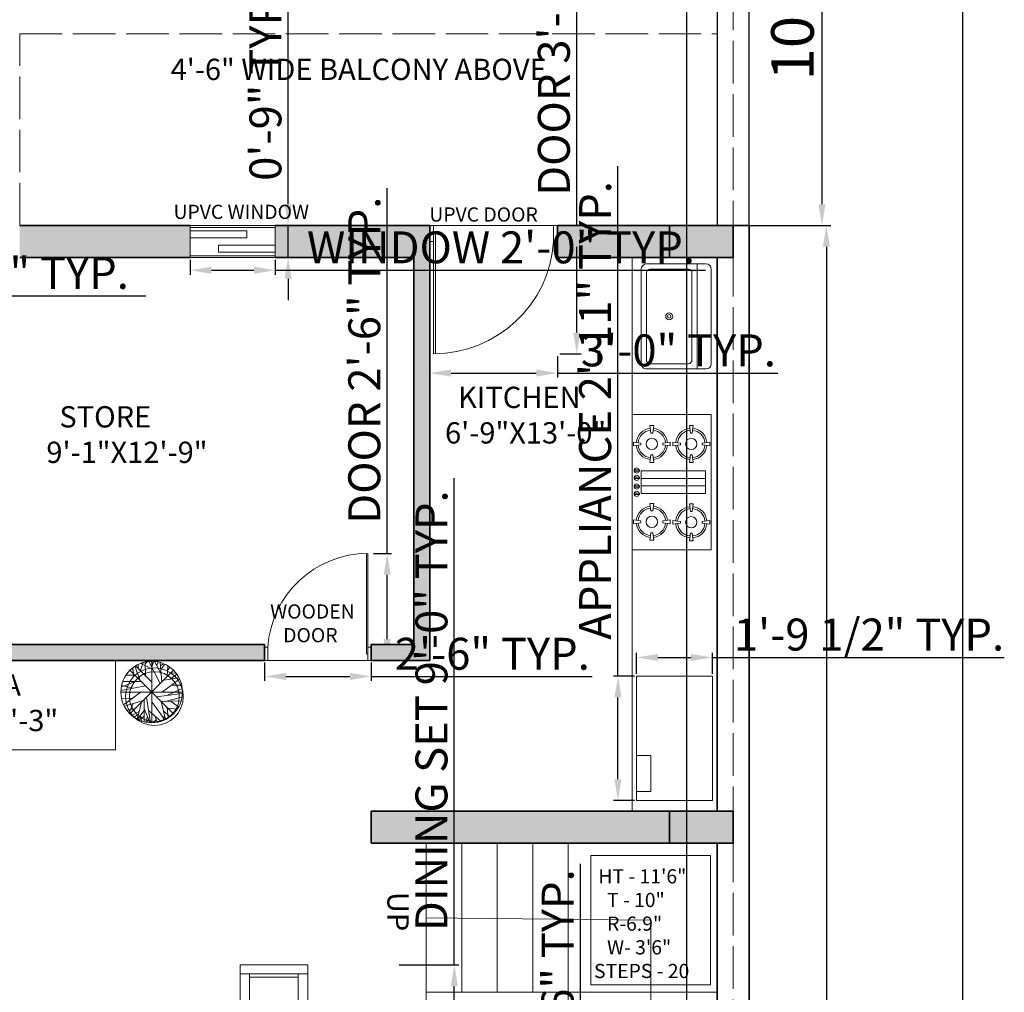
# Model space of a CAD drawing. Units: millimetres. Extents: x 595116 to 630915, y 909473 to 920225.
# Tile 125 of 134: x 629637 to 629914, y 919742 to 920016. Entities that reach past the tile are written whole.
import ezdxf

# ---------------------------------------------------------------- set-up
doc = ezdxf.new("R2010")
doc.units = ezdxf.units.MM
doc.linetypes.add('ACAD_ISO02W100', pattern=[15, 12, -3])
for name, color, linetype, lineweight in [('A-ANNO-SYMB', 7, 'Continuous', 18), ('A-AREA-IDEN', 7, 'Continuous', 20), ('A-EQPM', 8, 'Continuous', 13), ('A-FLOR-FIXT', 9, 'Continuous', 18), ('A-FLOR-OVHD', 253, 'ACAD_ISO02W100', 13), ('A-FLOR-STRS-HIDN', 142, 'ACAD_ISO02W100', 13), ('A-FURN', 32, 'Continuous', 18), ('A-WALL', 1, 'Continuous', 35), ('A-WALL-PATT', 8, 'Continuous', 13), ('C-PROP', 7, 'Continuous', 25), ('C-PROP-REF', 240, 'ACAD_ISO02W100', 13), ('Column', 6, 'Continuous', 35), ('Dimension', 3, 'Continuous', 18), ('Doors', 31, 'Continuous', 20), ('L-PLNT', 85, 'Continuous', 13), ('STAIR CASE', 142, 'Continuous', 20), ('Text', 7, 'Continuous', 18), ('Windows', 33, 'Continuous', 18)]:
    doc.layers.add(name, color=color, linetype=linetype, lineweight=lineweight)
doc.styles.get("Standard").update_dxf_attribs({"font": 'arial.ttf'})
doc.dimstyles.new('ISO-25', dxfattribs={"dimtxt": 9, "dimasz": 6, "dimexe": 1.25, "dimexo": 0.625, "dimtad": 1, "dimlunit": 4, "dimtxsty": 'Standard', "dimcen": 2.5, "dimadec": 0, "dimazin": 0, "dimtfac": 1, "dimtmove": 0, "dimatfit": 3, "dimfxl": 1, "dimarcsym": 0})

# ---------------------------------------------------------------- blocks, each defined once
blk = doc.blocks.new('KWD')
for points in [[(629753.63, 919957.93), (629752.54, 919957.93), (629752.54, 919953.43), (629753.63, 919953.43)], [(629787.45, 919957.93), (629787.45, 919953.43), (629788.54, 919953.43), (629788.54, 919957.93)]]:
    blk.add_lwpolyline(points, close=True)
blk.add_lwpolyline([(629753.63, 919921.79), (629753.63, 919955.68), (629754.13, 919955.68), (629754.13, 919921.8)])
blk.add_arc((629753.64, 919955.68), 33.88, 269.99, 356.196)
blk = doc.blocks.new('DS')
blk.add_lwpolyline([(630069.78, 919993.92), (630069.78, 919965.68), (630069.37, 919965.68), (630069.37, 919993.91)])
for points in [[(630041.6, 919963.81), (630041.6, 919967.56), (630040.69, 919967.56), (630040.69, 919963.81)], [(630069.78, 919963.81), (630070.69, 919963.81), (630070.69, 919967.56), (630069.78, 919967.56)]]:
    blk.add_lwpolyline(points, close=True)
blk.add_arc((630069.78, 919965.69), 28.24, 89.99, 176.196)
blk = doc.blocks.new('DINING')
for p, q in [((630176.61, 919568.69), (630176.61, 919601.05)), ((630176.61, 919601.05), (630208.41, 919601.05)), ((630208.41, 919601.05), (630208.41, 919568.69)), ((630176.61, 919596.78), (630208.41, 919596.78)), ((630181.05, 919571.76), (630181.05, 919596.78)), ((630181.05, 919595.21), (630203.97, 919595.21)), ((630203.97, 919571.76), (630203.97, 919596.78)), ((630176.61, 919570.82), (630180.11, 919570.82)), ((630208.41, 919570.82), (630204.91, 919570.82)), ((630163.47, 919568.69), (630222.04, 919568.69)), ((630163.47, 919453.21), (630163.47, 919568.69)), ((630164.11, 919568.05), (630221.39, 919568.05)), ((630164.11, 919453.85), (630164.11, 919568.05)), ((630221.39, 919568.05), (630221.39, 919453.85)), ((630222.04, 919568.69), (630222.04, 919453.21)), ((630163.47, 919544.57), (630135.12, 919544.57)), ((630135.12, 919544.57), (630135.12, 919519)), ((630137.93, 919544.57), (630137.93, 919519)), ((630138.72, 919544.57), (630138.72, 919519)), ((630222.04, 919544.57), (630250.39, 919544.57)), ((630246.79, 919544.57), (630246.79, 919519)), ((630247.58, 919544.57), (630247.58, 919519)), ((630250.39, 919544.57), (630250.39, 919519)), ((630135.12, 919519), (630163.47, 919519)), ((630250.39, 919519), (630222.04, 919519)), ((630163.47, 919503.52), (630135.12, 919503.52)), ((630135.12, 919503.52), (630135.12, 919477.96)), ((630137.93, 919503.52), (630137.93, 919477.96)), ((630138.72, 919503.52), (630138.72, 919477.96)), ((630222.04, 919503.52), (630250.39, 919503.52)), ((630246.79, 919503.52), (630246.79, 919477.96)), ((630247.58, 919503.52), (630247.58, 919477.96)), ((630250.39, 919503.52), (630250.39, 919477.96)), ((630135.12, 919477.96), (630163.47, 919477.96)), ((630250.39, 919477.96), (630222.04, 919477.96)), ((630222.04, 919453.21), (630163.47, 919453.21)), ((630221.39, 919453.85), (630164.11, 919453.85)), ((630176.61, 919453.21), (630176.61, 919420.86)), ((630176.61, 919451.09), (630180.11, 919451.09)), ((630208.41, 919451.09), (630204.91, 919451.09)), ((630208.41, 919420.86), (630208.41, 919453.21)), ((630181.05, 919450.14), (630181.05, 919425.13)), ((630203.97, 919450.14), (630203.97, 919425.13)), ((630176.61, 919425.13), (630208.41, 919425.13)), ((630181.05, 919426.7), (630203.97, 919426.7)), ((630176.61, 919420.86), (630208.41, 919420.86))]:
    blk.add_line(p, q)
for centre, start, end in [((630180.11, 919571.76), 270, 0), ((630204.91, 919571.76), 180, 270), ((630180.11, 919450.14), 0, 90), ((630204.91, 919450.14), 90, 180)]:
    blk.add_arc(centre, 0.945, start, end)
blk = doc.blocks.new('A$C57CF26DA')
for p, q in [((0, 0), (0, 420)), ((720, 420), (0, 420)), ((720, 0), (720, 420)), ((166.9, 413), (146.9, 413)), ((146.9, 413), (151.9, 373)), ((151.9, 373), (161.9, 373)), ((161.9, 373), (166.9, 413)), ((300, 390.9), (300, 49.1)), ((300, 390.9), (420, 390.9)), ((340, 390.9), (340, 49.1)), ((380, 390.9), (380, 49.1)), ((420, 390.9), (420, 49.1)), ((583.6, 413), (563.6, 413)), ((563.6, 413), (568.6, 373)), ((568.6, 373), (578.6, 373)), ((578.6, 373), (583.6, 413)), ((98.9, 320), (58.9, 325)), ((58.9, 325), (58.9, 305)), ((98.9, 310), (98.9, 320)), ((254.8, 325), (214.8, 320)), ((214.8, 320), (214.8, 310)), ((254.8, 305), (254.8, 325)), ((515.6, 320), (475.6, 325)), ((475.6, 325), (475.6, 305)), ((515.6, 310), (515.6, 320)), ((671.6, 325), (631.6, 320)), ((631.6, 320), (631.6, 310)), ((671.6, 305), (671.6, 325)), ((58.9, 305), (98.9, 310)), ((214.8, 310), (254.8, 305)), ((475.6, 305), (515.6, 310)), ((631.6, 310), (671.6, 305)), ((151.9, 257), (146.9, 217)), ((146.9, 217), (166.9, 217)), ((161.9, 257), (151.9, 257)), ((166.9, 217), (161.9, 257)), ((568.6, 257), (563.6, 217)), ((563.6, 217), (583.6, 217)), ((578.6, 257), (568.6, 257)), ((583.6, 217), (578.6, 257)), ((166.9, 203), (146.9, 203)), ((146.9, 203), (151.9, 163)), ((151.9, 163), (161.9, 163)), ((161.9, 163), (166.9, 203)), ((581.1, 203), (561.1, 203)), ((561.1, 203), (566.1, 163)), ((566.1, 163), (576.1, 163)), ((576.1, 163), (581.1, 203)), ((98.9, 110), (58.9, 115)), ((58.9, 115), (58.9, 95)), ((98.9, 100), (98.9, 110)), ((254.8, 115), (214.8, 110)), ((214.8, 110), (214.8, 100)), ((254.8, 95), (254.8, 115)), ((513.1, 110), (473.1, 115)), ((473.1, 115), (473.1, 95)), ((513.1, 100), (513.1, 110)), ((669, 115), (629, 110)), ((629, 110), (629, 100)), ((669, 95), (669, 115)), ((58.9, 95), (98.9, 100)), ((214.8, 100), (254.8, 95)), ((473.1, 95), (513.1, 100)), ((629, 100), (669, 95)), ((151.9, 47), (146.9, 7)), ((146.9, 7), (166.9, 7)), ((161.9, 47), (151.9, 47)), ((166.9, 7), (161.9, 47)), ((301.5, 38.7), (294.7, 38.7)), ((294.7, 38.7), (294.7, 11.3)), ((294.7, 11.3), (301.5, 11.3)), ((420, 49.1), (300, 49.1)), ((301.5, 11.3), (301.5, 38.7)), ((340.5, 38.7), (333.7, 38.7)), ((333.7, 38.7), (333.7, 11.3)), ((333.7, 11.3), (340.5, 11.3)), ((340.5, 11.3), (340.5, 38.7)), ((379.7, 11.3), (379.7, 38.7)), ((379.7, 38.7), (386.5, 38.7)), ((386.5, 11.3), (379.7, 11.3)), ((386.5, 38.7), (386.5, 11.3)), ((418.7, 11.3), (418.7, 38.7)), ((418.7, 38.7), (425.5, 38.7)), ((425.5, 11.3), (418.7, 11.3)), ((425.5, 38.7), (425.5, 11.3)), ((566.1, 47), (561.1, 7)), ((561.1, 7), (581.1, 7)), ((576.1, 47), (566.1, 47)), ((581.1, 7), (576.1, 47)), ((720, 0), (0, 0))]:
    blk.add_line(p, q)
for centre in [(156.9, 315), (573.6, 315), (156.9, 105), (571.1, 105)]:
    blk.add_circle(centre, 30)
for centre, radius, start, end in [((156.9, 315), 83, 95.5849, 174.4151), ((156.9, 315), 73, 95.3738, 174.6262), ((156.9, 315), 73, 5.3738, 84.6262), ((156.9, 315), 83, 5.5849, 84.4151), ((573.6, 315), 83, 95.5849, 174.4151), ((573.6, 315), 73, 95.3738, 174.6262), ((573.6, 315), 73, 5.3738, 84.6262), ((573.6, 315), 83, 5.5849, 84.4151), ((156.9, 315), 83, 185.5849, 264.4151), ((156.9, 315), 73, 185.3738, 264.6262), ((156.9, 315), 73, 275.3738, 354.6262), ((156.9, 315), 83, 275.5849, 354.4151), ((573.6, 315), 83, 185.5849, 264.4151), ((573.6, 315), 73, 185.3738, 264.6262), ((573.6, 315), 73, 275.3738, 354.6262), ((573.6, 315), 83, 275.5849, 354.4151), ((156.9, 105), 83, 95.5849, 174.4151), ((156.9, 105), 73, 95.3738, 174.6262), ((156.9, 105), 73, 5.3738, 84.6262), ((156.9, 105), 83, 5.5849, 84.4151), ((571.1, 105), 83, 95.5849, 174.4151), ((571.1, 105), 73, 95.3738, 174.6262), ((571.1, 105), 73, 5.3738, 84.6262), ((571.1, 105), 83, 5.5849, 84.4151), ((156.9, 105), 83, 185.5849, 264.4151), ((156.9, 105), 73, 185.3738, 264.6262), ((156.9, 105), 73, 275.3738, 354.6262), ((156.9, 105), 83, 275.5849, 354.4151), ((571.1, 105), 83, 185.5849, 264.4151), ((571.1, 105), 73, 185.3738, 264.6262), ((571.1, 105), 73, 275.3738, 354.6262), ((571.1, 105), 83, 275.5849, 354.4151), ((298.1, 25), 13.7, 104.4775, 255.5225), ((298.1, 25), 13.7, 284.4775, 75.5225), ((337.1, 25), 13.7, 104.4775, 255.5225), ((337.1, 25), 13.7, 284.4775, 75.5225), ((383.1, 25), 13.7, 104.4775, 255.5225), ((383.1, 25), 13.7, 284.4775, 75.5225), ((422.1, 25), 13.7, 104.4775, 255.5225), ((422.1, 25), 13.7, 284.4775, 75.5225)]:
    blk.add_arc(centre, radius, start, end)
blk = doc.blocks.new('Sink-single - 30 in top')
blk.add_line((-15, -3.999996), (15, -3.999996))
for points in [[(-13.5, 0), (13.5, 0)], [(-15, -18.499996), (-15, -1.5)], [(15, -1.5), (15, -18.499996)], [(-12.5, -5.499996), (12.5, -5.499996)], [(-13.5, -17.499996), (-13.5, -6.499996)], [(13.5, -6.499996), (13.5, -17.499996)], [(12.5, -18.499996), (-12.5, -18.499996)], [(13.5, -19.999996), (-13.5, -19.999996)]]:
    blk.add_lwpolyline(points)
for radius in [1, 0.5]:
    blk.add_circle((0, -11.999996), radius)
for centre, radius, start, end in [((-13.5, -1.5), 1.5, 90, 180), ((13.5, -1.5), 1.5, 0, 90), ((-12.5, -6.499996), 1, 90, 180), ((12.5, -6.499996), 1, 0, 90), ((-13.5, -18.499996), 1.5, 180, 270), ((-12.5, -17.499996), 1, 180, 270), ((12.5, -17.499996), 1, 270, 0), ((13.5, -18.499996), 1.5, 270, 0)]:
    blk.add_arc(centre, radius, start, end)
blk = doc.blocks.new('*D121')
at = {"layer": 'Defpoints', "color": 0, "transparency": 16777216}
for p in [(629838.04, 920084.93), (629838.04, 919957.93), (629863.03, 919957.93)]:
    blk.add_point(p, dxfattribs=at)
at = {"layer": 'Dimension', "color": 0, "lineweight": -2, "transparency": 16777216}
for p, q in [((629838.67, 920084.93), (629864.28, 920084.93)), ((629863.03, 920078.93), (629863.03, 919963.93)), ((629838.67, 919957.93), (629864.28, 919957.93))]:
    blk.add_line(p, q, dxfattribs=at)
at = {"layer": 'Dimension', "color": 0, "transparency": 16777216}
for points in [[(629862.03, 920078.93), (629864.03, 920078.93), (629863.03, 920084.93)], [(629862.03, 919963.93), (629864.03, 919963.93), (629863.03, 919957.93)]]:
    blk.add_solid(points, dxfattribs=at)
at = {"layer": 'Dimension', "color": 0, "transparency": 16777216, "insert": (629856.28, 920021.43), "char_height": 12, "attachment_point": 5, "rotation": 90}
blk.add_mtext('10\'-7"', dxfattribs=at)
blk = doc.blocks.new('*D122')
at = {"layer": 'Defpoints', "color": 0, "transparency": 16777216}
for p in [(629862.34, 919957.93), (629854.28, 919369.93), (629864.28, 919369.93)]:
    blk.add_point(p, dxfattribs=at)
at = {"layer": 'Dimension', "color": 0, "lineweight": -2, "transparency": 16777216}
for p, q in [((629862.97, 919957.93), (629865.53, 919957.93)), ((629864.28, 919951.93), (629864.28, 919375.93)), ((629854.9, 919369.93), (629865.53, 919369.93))]:
    blk.add_line(p, q, dxfattribs=at)
at = {"layer": 'Dimension', "color": 0, "transparency": 16777216}
for points in [[(629863.28, 919951.93), (629865.28, 919951.93), (629864.28, 919957.93)], [(629863.28, 919375.93), (629865.28, 919375.93), (629864.28, 919369.93)]]:
    blk.add_solid(points, dxfattribs=at)
at = {"layer": 'Dimension', "color": 0, "transparency": 16777216, "insert": (629857.53, 919663.93), "char_height": 12, "attachment_point": 5, "rotation": 90}
blk.add_mtext("49'", dxfattribs=at)
blk = doc.blocks.new('*D124')
at = {"layer": 'Defpoints', "color": 0, "transparency": 16777216}
for p in [(629865.75, 920084.93), (629865.75, 919141.93), (629902.57, 919141.93)]:
    blk.add_point(p, dxfattribs=at)
at = {"layer": 'Dimension', "color": 0, "lineweight": -2, "transparency": 16777216}
for p, q in [((629866.37, 920084.93), (629903.82, 920084.93)), ((629902.57, 920078.93), (629902.57, 919147.93)), ((629866.37, 919141.93), (629903.82, 919141.93))]:
    blk.add_line(p, q, dxfattribs=at)
at = {"layer": 'Dimension', "color": 0, "transparency": 16777216}
for points in [[(629901.57, 920078.93), (629903.57, 920078.93), (629902.57, 920084.93)], [(629901.57, 919147.93), (629903.57, 919147.93), (629902.57, 919141.93)]]:
    blk.add_solid(points, dxfattribs=at)
at = {"layer": 'Dimension', "color": 0, "transparency": 16777216, "insert": (629897.35, 919613.43), "char_height": 9, "attachment_point": 5, "rotation": 90}
blk.add_mtext('78\'-7"', dxfattribs=at)
blk = doc.blocks.new('POTTED-PLANT')
for p, q in [((3.96, 16.73), (5.31, 12.84)), ((4.16, 16.82), (8.64, 12.35)), ((4.85, 16.17), (4.88, 17.22)), ((5.49, 15.52), (6.28, 17.77)), ((5.61, 17.51), (8.67, 15.94)), ((6.86, 17.38), (7.52, 18.03)), ((6.89, 14.08), (6.86, 17.93)), ((7.9, 18.06), (11.06, 11.86)), ((9.02, 17.38), (8.46, 18.1)), ((8.67, 18.11), (8.67, 0.76)), ((8.74, 16.47), (9.2, 18.06)), ((11.32, 14.57), (9.46, 18.06)), ((10.09, 16.89), (10.53, 17.9)), ((11.52, 12.26), (11.04, 17.77)), ((11.14, 16.82), (12.03, 17.41)), ((11.24, 15.75), (12.36, 17.28)), ((13.25, 16.79), (13.05, 13.86)), ((1.47, 14.18), (3.93, 14.18)), ((14.75, 15.51), (2.6, 3.36)), ((14.75, 3.36), (2.6, 15.51)), ((2.87, 15.88), (3.4, 15.68)), ((3.32, 16.24), (3.58, 14.57)), ((13.17, 15.58), (13.86, 16.4)), ((13.91, 13.07), (15.74, 14.51)), ((14.04, 14.8), (15.41, 14.87)), ((0.04, 9.84), (6.94, 11.18)), ((4.01, 12.42), (0.12, 10.79)), ((0.19, 11.28), (3.48, 10.53)), ((0.57, 12.45), (5.66, 12.45)), ((16.53, 13.1), (11.7, 9.48)), ((12.05, 12.81), (16.38, 13.4)), ((14.24, 11.38), (17.09, 11.41)), ((0, 9.44), (17.35, 9.44)), ((0.78, 5.86), (5.74, 9.45)), ((10.02, 8.11), (17.3, 9.03)), ((12.92, 8.47), (17.27, 10.46)), ((0.22, 7.66), (3.4, 7.75)), ((0.98, 5.47), (6.25, 7.04)), ((3.48, 6.19), (2.31, 3.58)), ((5.79, 6.51), (4.54, 1.82)), ((6.53, 7.26), (6.56, 1.1)), ((7.22, 7.98), (8.31, 0.8)), ((8.67, 6.68), (12.41, 1.65)), ((11.37, 6.74), (12.54, 1.72)), ((11.39, 6.74), (16.97, 6.94)), ((12.49, 6.77), (17.19, 8.01)), ((14.19, 6.81), (16.25, 5.24)), ((3.99, 4.75), (1.72, 4.29)), ((5.1, 3.97), (3.07, 2.83)), ((4.88, 3.09), (3.65, 2.4)), ((6.56, 4.2), (4.67, 1.78)), ((5.56, 2.86), (5.79, 1.33)), ((6.56, 4.78), (8.11, 0.84)), ((7.78, 4.2), (11.26, 1.2)), ((11.98, 4.16), (13.78, 2.43)), ((12.26, 2.96), (12, 1.49)), ((13.07, 5.08), (13.35, 2.21)), ((13.22, 4.91), (15.85, 4.62)), ((6.56, 2.6), (5.05, 1.59)), ((7.45, 2.57), (7.01, 0.97)), ((7.75, 1.82), (7.32, 0.93)), ((9.89, 1.75), (9.23, 0.84)), ((9.53, 2.7), (10.2, 0.97))]:
    blk.add_line(p, q)
for centre, radius in [((8.67, 9.44), 8.67), ((9.43, 8.14), 8.14), ((9.43, 8.14), 7.03)]:
    blk.add_circle(centre, radius)
blk = doc.blocks.new('WIN-UPVC-2FT')
for p, q in [((0, 9), (0, 0)), ((0, 9), (24, 9)), ((24, 9), (24, 0)), ((0, 7.5), (16, 7.5)), ((0, 0), (24, 0))]:
    blk.add_line(p, q)
blk.add_lwpolyline([(0, 8.46), (24, 8.46), (24, 0.48), (0, 0.48)], close=True)
for points in [[(0, 5.5), (16, 5.5), (16, 7.5)], [(24, 1.5), (8, 1.5), (8, 3.5), (24, 3.5)]]:
    blk.add_lwpolyline(points)
blk = doc.blocks.new('KITCHEN-APPLIANCE')
for points in [[(0, 35.07), (21.33, 35.07), (21.33, 0), (0, 0)], [(0, 12.66), (4.02, 12.66), (4.02, 2.57), (0, 2.57)]]:
    blk.add_lwpolyline(points, close=True)
blk = doc.blocks.new('COLUMN-RECT-18X9')
h = blk.add_hatch(color=256)
h.dxf.hatch_style = 1
h.paths.add_polyline_path([(18, 9), (0, 9), (0, 0), (18, 0)])
blk.add_lwpolyline([(0, 9), (18, 9), (18, 0), (0, 0)], close=True)
blk = doc.blocks.new('COLUMN-RECT-18X9-B')
h = blk.add_hatch(color=256)
h.dxf.hatch_style = 1
h.paths.add_polyline_path([(18, 0), (18, 9), (0, 9), (0, 0)])
blk.add_lwpolyline([(0, 9), (18, 9), (18, 0), (0, 0)], close=True)
blk = doc.blocks.new('*D160')
at = {"layer": 'Defpoints', "color": 0, "transparency": 16777216}
for p in [(629788.54, 919957.93), (629793.96, 919957.93), (629788.54, 919921.79)]:
    blk.add_point(p, dxfattribs=at)
at = {"layer": 'Dimension', "color": 0, "lineweight": -2, "transparency": 16777216}
for p, q in [((629793.96, 919957.93), (629793.96, 920060.8)), ((629789.17, 919957.93), (629795.21, 919957.93)), ((629793.96, 919927.79), (629793.96, 919951.93)), ((629789.17, 919921.79), (629795.21, 919921.79))]:
    blk.add_line(p, q, dxfattribs=at)
at = {"layer": 'Dimension', "color": 0, "transparency": 16777216}
for points in [[(629792.96, 919951.93), (629794.96, 919951.93), (629793.96, 919957.93)], [(629792.96, 919927.79), (629794.96, 919927.79), (629793.96, 919921.79)]]:
    blk.add_solid(points, dxfattribs=at)
at = {"layer": 'Dimension', "color": 0, "transparency": 16777216, "insert": (629788.68, 920012.36), "char_height": 9, "attachment_point": 5, "rotation": 90}
blk.add_mtext('DOOR 3\'-0" TYP.', dxfattribs=at)
blk = doc.blocks.new('*D161')
at = {"layer": 'Defpoints', "color": 0, "transparency": 16777216}
for p in [(629752.54, 919921.79), (629788.54, 919921.79), (629788.54, 919916.37)]:
    blk.add_point(p, dxfattribs=at)
at = {"layer": 'Dimension', "color": 0, "lineweight": -2, "transparency": 16777216}
for p, q in [((629752.54, 919921.16), (629752.54, 919915.12)), ((629788.54, 919921.16), (629788.54, 919915.12)), ((629758.54, 919916.37), (629782.54, 919916.37)), ((629788.54, 919916.37), (629850.64, 919916.37))]:
    blk.add_line(p, q, dxfattribs=at)
at = {"layer": 'Dimension', "color": 0, "transparency": 16777216}
for points in [[(629758.54, 919917.37), (629758.54, 919915.37), (629752.54, 919916.37)], [(629782.54, 919917.37), (629782.54, 919915.37), (629788.54, 919916.37)]]:
    blk.add_solid(points, dxfattribs=at)
at = {"layer": 'Dimension', "color": 0, "transparency": 16777216, "insert": (629822.59, 919921.59), "char_height": 9, "attachment_point": 5}
blk.add_mtext('3\'-0" TYP.', dxfattribs=at)
blk = doc.blocks.new('*D164')
at = {"layer": 'Defpoints', "color": 0, "transparency": 16777216}
for p in [(629736.04, 919865.54), (629740.56, 919865.54), (629736.04, 919835.43)]:
    blk.add_point(p, dxfattribs=at)
at = {"layer": 'Dimension', "color": 0, "lineweight": -2, "transparency": 16777216}
for p, q in [((629740.56, 919865.54), (629740.56, 919968.42)), ((629736.67, 919865.54), (629741.81, 919865.54)), ((629740.56, 919841.43), (629740.56, 919859.54)), ((629736.67, 919835.43), (629741.81, 919835.43))]:
    blk.add_line(p, q, dxfattribs=at)
at = {"layer": 'Dimension', "color": 0, "transparency": 16777216}
for points in [[(629739.56, 919859.54), (629741.56, 919859.54), (629740.56, 919865.54)], [(629739.56, 919841.43), (629741.56, 919841.43), (629740.56, 919835.43)]]:
    blk.add_solid(points, dxfattribs=at)
at = {"layer": 'Dimension', "color": 0, "transparency": 16777216, "insert": (629735.28, 919919.98), "char_height": 9, "attachment_point": 5, "rotation": 90}
blk.add_mtext('DOOR 2\'-6" TYP.', dxfattribs=at)
blk = doc.blocks.new('*D165')
at = {"layer": 'Defpoints', "color": 0, "transparency": 16777216}
for p in [(629706.04, 919835.43), (629736.04, 919835.43), (629736.04, 919830.91)]:
    blk.add_point(p, dxfattribs=at)
at = {"layer": 'Dimension', "color": 0, "lineweight": -2, "transparency": 16777216}
for p, q in [((629706.04, 919834.8), (629706.04, 919829.66)), ((629736.04, 919834.8), (629736.04, 919829.66)), ((629712.04, 919830.91), (629730.04, 919830.91)), ((629736.04, 919830.91), (629798.3, 919830.91))]:
    blk.add_line(p, q, dxfattribs=at)
at = {"layer": 'Dimension', "color": 0, "transparency": 16777216}
for points in [[(629712.04, 919831.91), (629712.04, 919829.91), (629706.04, 919830.91)], [(629730.04, 919831.91), (629730.04, 919829.91), (629736.04, 919830.91)]]:
    blk.add_solid(points, dxfattribs=at)
at = {"layer": 'Dimension', "color": 0, "transparency": 16777216, "insert": (629770.17, 919836.13), "char_height": 9, "attachment_point": 5}
blk.add_mtext('2\'-6" TYP.', dxfattribs=at)
blk = doc.blocks.new('*D180')
at = {"layer": 'Defpoints', "color": 0, "transparency": 16777216}
for p in [(629743.29, 919749.69), (629759.47, 919749.69), (629743.29, 919641.85)]:
    blk.add_point(p, dxfattribs=at)
at = {"layer": 'Dimension', "color": 0, "lineweight": -2, "transparency": 16777216}
for p, q in [((629759.47, 919749.69), (629759.47, 919886.8)), ((629743.92, 919749.69), (629760.72, 919749.69)), ((629759.47, 919647.85), (629759.47, 919743.69)), ((629743.92, 919641.85), (629760.72, 919641.85))]:
    blk.add_line(p, q, dxfattribs=at)
at = {"layer": 'Dimension', "color": 0, "transparency": 16777216}
for points in [[(629758.47, 919743.69), (629760.47, 919743.69), (629759.47, 919749.69)], [(629758.47, 919647.85), (629760.47, 919647.85), (629759.47, 919641.85)]]:
    blk.add_solid(points, dxfattribs=at)
at = {"layer": 'Dimension', "color": 0, "transparency": 16777216, "insert": (629754.19, 919821.24), "char_height": 9, "attachment_point": 5, "rotation": 90}
blk.add_mtext('DINING SET 9\'-0" TYP.', dxfattribs=at)
blk = doc.blocks.new('*D192')
at = {"layer": 'Defpoints', "color": 0, "transparency": 16777216}
for p in [(629426.04, 919948.93), (629498.04, 919948.93), (629498.04, 919938.13)]:
    blk.add_point(p, dxfattribs=at)
at = {"layer": 'Dimension', "color": 0, "lineweight": -2, "transparency": 16777216}
for p, q in [((629426.04, 919948.3), (629426.04, 919936.88)), ((629498.04, 919948.3), (629498.04, 919936.88)), ((629432.04, 919938.13), (629492.04, 919938.13)), ((629498.04, 919938.13), (629672.56, 919938.13))]:
    blk.add_line(p, q, dxfattribs=at)
at = {"layer": 'Dimension', "color": 0, "transparency": 16777216}
for points in [[(629432.04, 919939.13), (629432.04, 919937.13), (629426.04, 919938.13)], [(629492.04, 919939.13), (629492.04, 919937.13), (629498.04, 919938.13)]]:
    blk.add_solid(points, dxfattribs=at)
at = {"layer": 'Dimension', "color": 0, "transparency": 16777216, "insert": (629588.3, 919943.41), "char_height": 9, "attachment_point": 5}
blk.add_mtext('SLIDING WINDOW 6\'-0" TYP.', dxfattribs=at)
blk = doc.blocks.new('*D196')
at = {"layer": 'Defpoints', "color": 0, "transparency": 16777216}
for p in [(629685.04, 919948.93), (629709.04, 919948.93), (629709.04, 919945.33)]:
    blk.add_point(p, dxfattribs=at)
at = {"layer": 'Dimension', "color": 0, "lineweight": -2, "transparency": 16777216}
for p, q in [((629685.04, 919948.3), (629685.04, 919944.08)), ((629709.04, 919948.3), (629709.04, 919944.08)), ((629691.04, 919945.33), (629703.04, 919945.33)), ((629709.04, 919945.33), (629830.18, 919945.33))]:
    blk.add_line(p, q, dxfattribs=at)
at = {"layer": 'Dimension', "color": 0, "transparency": 16777216}
for points in [[(629691.04, 919946.33), (629691.04, 919944.33), (629685.04, 919945.33)], [(629703.04, 919946.33), (629703.04, 919944.33), (629709.04, 919945.33)]]:
    blk.add_solid(points, dxfattribs=at)
at = {"layer": 'Dimension', "color": 0, "transparency": 16777216, "insert": (629772.61, 919950.61), "char_height": 9, "attachment_point": 5}
blk.add_mtext('WINDOW 2\'-0" TYP.', dxfattribs=at)
blk = doc.blocks.new('*D197')
at = {"layer": 'Defpoints', "color": 0, "transparency": 16777216}
for p in [(629709.04, 919957.93), (629712.64, 919957.93), (629709.04, 919948.93)]:
    blk.add_point(p, dxfattribs=at)
at = {"layer": 'Dimension', "color": 0, "lineweight": -2, "transparency": 16777216}
for p, q in [((629712.64, 919963.93), (629712.64, 920026.04)), ((629709.67, 919957.93), (629713.89, 919957.93)), ((629712.64, 919948.93), (629712.64, 919957.93)), ((629709.67, 919948.93), (629713.89, 919948.93)), ((629712.64, 919942.93), (629712.64, 919936.93))]:
    blk.add_line(p, q, dxfattribs=at)
at = {"layer": 'Dimension', "color": 0, "transparency": 16777216}
for points in [[(629711.64, 919963.93), (629713.64, 919963.93), (629712.64, 919957.93)], [(629711.64, 919942.93), (629713.64, 919942.93), (629712.64, 919948.93)]]:
    blk.add_solid(points, dxfattribs=at)
at = {"layer": 'Dimension', "color": 0, "transparency": 16777216, "insert": (629707.42, 919997.98), "char_height": 9, "attachment_point": 5, "rotation": 90}
blk.add_mtext('0\'-9" TYP.', dxfattribs=at)
blk = doc.blocks.new('*D200')
at = {"layer": 'Defpoints', "color": 0, "transparency": 16777216}
for p in [(629805.57, 919831), (629810.83, 919831), (629810.83, 919795.93)]:
    blk.add_point(p, dxfattribs=at)
at = {"layer": 'Dimension', "color": 0, "lineweight": -2, "transparency": 16777216}
for p, q in [((629805.57, 919831), (629805.57, 919974.69)), ((629810.21, 919831), (629804.32, 919831)), ((629805.57, 919801.93), (629805.57, 919825)), ((629810.21, 919795.93), (629804.32, 919795.93))]:
    blk.add_line(p, q, dxfattribs=at)
at = {"layer": 'Dimension', "color": 0, "transparency": 16777216}
for points in [[(629804.57, 919825), (629806.57, 919825), (629805.57, 919831)], [(629804.57, 919801.93), (629806.57, 919801.93), (629805.57, 919795.93)]]:
    blk.add_solid(points, dxfattribs=at)
at = {"layer": 'Dimension', "color": 0, "transparency": 16777216, "insert": (629800.29, 919905.85), "char_height": 9, "attachment_point": 5, "rotation": 90}
blk.add_mtext('APPLIANCE 2\'-11" TYP.', dxfattribs=at)
blk = doc.blocks.new('*D201')
at = {"layer": 'Defpoints', "color": 0, "transparency": 16777216}
for p in [(629832.16, 919836.26), (629810.83, 919831), (629832.16, 919831)]:
    blk.add_point(p, dxfattribs=at)
at = {"layer": 'Dimension', "color": 0, "lineweight": -2, "transparency": 16777216}
for p, q in [((629810.83, 919831.62), (629810.83, 919837.51)), ((629816.83, 919836.26), (629826.16, 919836.26)), ((629832.16, 919831.62), (629832.16, 919837.51)), ((629832.16, 919836.26), (629914.39, 919836.26))]:
    blk.add_line(p, q, dxfattribs=at)
at = {"layer": 'Dimension', "color": 0, "transparency": 16777216}
for points in [[(629816.83, 919837.26), (629816.83, 919835.26), (629810.83, 919836.26)], [(629826.16, 919837.26), (629826.16, 919835.26), (629832.16, 919836.26)]]:
    blk.add_solid(points, dxfattribs=at)
at = {"layer": 'Dimension', "color": 0, "transparency": 16777216, "insert": (629876.28, 919841.54), "char_height": 9, "attachment_point": 5}
blk.add_mtext('1\'-9 1/2" TYP.', dxfattribs=at)
blk = doc.blocks.new('*D208')
at = {"layer": 'Defpoints', "color": 0, "transparency": 16777216}
for p in [(629792.3, 919687.12), (629794.99, 919687.12), (629792.3, 919669.18)]:
    blk.add_point(p, dxfattribs=at)
at = {"layer": 'Dimension', "color": 0, "lineweight": -2, "transparency": 16777216}
for p, q in [((629794.99, 919687.12), (629794.99, 919778.12)), ((629792.93, 919687.12), (629796.24, 919687.12)), ((629794.99, 919675.18), (629794.99, 919681.12)), ((629792.93, 919669.18), (629796.24, 919669.18))]:
    blk.add_line(p, q, dxfattribs=at)
at = {"layer": 'Dimension', "color": 0, "transparency": 16777216}
for points in [[(629793.99, 919681.12), (629795.99, 919681.12), (629794.99, 919687.12)], [(629793.99, 919675.18), (629795.99, 919675.18), (629794.99, 919669.18)]]:
    blk.add_solid(points, dxfattribs=at)
at = {"layer": 'Dimension', "color": 0, "transparency": 16777216, "insert": (629789.71, 919735.62), "char_height": 9, "attachment_point": 5, "rotation": 90}
blk.add_mtext('POT 1\'-6" TYP.', dxfattribs=at)
blk = doc.blocks.new('*D220')
at = {"layer": 'Defpoints', "color": 0, "transparency": 16777216}
for p in [(629824.95, 920160.76), (629511.27, 919302.01), (629824.95, 919302.01)]:
    blk.add_point(p, dxfattribs=at)
at = {"layer": 'Dimension', "color": 0, "lineweight": -2, "transparency": 16777216}
for p, q in [((629511.27, 919302.63), (629511.27, 920162.01)), ((629517.27, 920160.76), (629818.95, 920160.76)), ((629824.95, 919302.63), (629824.95, 920162.01))]:
    blk.add_line(p, q, dxfattribs=at)
at = {"layer": 'Dimension', "color": 0, "transparency": 16777216}
for points in [[(629517.27, 920161.76), (629517.27, 920159.76), (629511.27, 920160.76)], [(629818.95, 920161.76), (629818.95, 920159.76), (629824.95, 920160.76)]]:
    blk.add_solid(points, dxfattribs=at)
at = {"layer": 'Dimension', "color": 0, "transparency": 16777216, "insert": (629668.11, 920166.03), "char_height": 9, "attachment_point": 5}
blk.add_mtext('26\'-1 1/2"', dxfattribs=at)

msp = doc.modelspace()

# ---------------------------------------------------------------- hatches: boundary and pattern name
at = {"layer": 'A-WALL-PATT'}
h = msp.add_hatch(color=256, dxfattribs=at)
h.dxf.hatch_style = 1
h.paths.add_polyline_path([(629685.041, 919957.928), (629637.041, 919957.928), (629637.041, 919948.928), (629685.041, 919948.928)])
h = msp.add_hatch(color=256, dxfattribs=at)
h.dxf.hatch_style = 1
h.paths.add_polyline_path([(629752.541, 919957.928), (629709.041, 919957.928), (629709.041, 919948.928), (629748.041, 919948.928), (629748.041, 919839.928), (629736.041, 919839.928), (629736.041, 919835.428), (629752.541, 919835.428)])
h = msp.add_hatch(color=256, dxfattribs=at)
h.dxf.hatch_style = 1
h.paths.add_polyline_path([(629820.041, 919957.928), (629788.541, 919957.928), (629788.541, 919948.928), (629820.041, 919948.928)])
h = msp.add_hatch(color=256, dxfattribs=at)
h.dxf.hatch_style = 1
h.paths.add_polyline_path([(629706.041, 919839.928), (629595.041, 919839.928), (629595.041, 919835.428), (629706.041, 919835.428)])
h = msp.add_hatch(color=256, dxfattribs=at)
h.dxf.hatch_style = 1
h.paths.add_polyline_path([(629820.041, 919792.928), (629736.041, 919792.928), (629736.041, 919783.928), (629820.041, 919783.928)])

# ---------------------------------------------------------------- linework, layer by layer
at = {"layer": 'A-ANNO-SYMB'}
for p, q in [((629751.541, 919762.928), (629814.804, 919762.246)), ((629814.804, 919762.246), (629814.804, 919711.928))]:
    msp.add_line(p, q, dxfattribs=at)
msp.add_lwpolyline([(629797.931, 919780.49), (629831.678, 919780.49), (629831.678, 919744.002), (629797.931, 919744.002)], close=True, dxfattribs=at)
at = {"layer": 'A-FLOR-FIXT'}
msp.add_line((629809.541, 919948.928), (629809.541, 919792.928), dxfattribs=at)
at = {"layer": 'A-FLOR-OVHD'}
for p, q in [((629637.041, 920011.928), (629833.541, 920011.928)), ((629637.041, 919957.928), (629637.041, 920011.928))]:
    msp.add_line(p, q, dxfattribs=at)
at = {"layer": 'A-FLOR-STRS-HIDN'}
msp.add_line((629751.541, 919741.928), (629751.541, 919651.928), dxfattribs=at)
at = {"layer": 'A-FURN'}
for p in [(629664.041, 919835.428), (629595.041, 919810.258)]:
    msp.add_line(p, (629664.041, 919810.258), dxfattribs=at)
at = {"layer": 'A-WALL'}
for p, q in [((629637.041, 919957.928), (629685.041, 919957.928)), ((629709.041, 919957.928), (629752.541, 919957.928)), ((629752.541, 919957.928), (629752.541, 919835.428)), ((629788.541, 919957.928), (629788.541, 919948.928)), ((629788.541, 919957.928), (629842.541, 919957.928)), ((629637.041, 919948.928), (629685.041, 919948.928)), ((629709.041, 919948.928), (629748.041, 919948.928)), ((629748.041, 919948.928), (629748.041, 919839.928)), ((629788.541, 919948.928), (629838.041, 919948.928)), ((629833.541, 919948.928), (629833.541, 919792.928)), ((629595.041, 919839.928), (629706.041, 919839.928)), ((629706.041, 919839.928), (629706.041, 919835.428)), ((629736.041, 919839.928), (629748.041, 919839.928)), ((629736.041, 919839.928), (629736.041, 919835.428)), ((629595.041, 919835.428), (629706.041, 919835.428)), ((629736.041, 919835.428), (629752.541, 919835.428)), ((629736.041, 919792.928), (629838.041, 919792.928)), ((629736.041, 919792.928), (629736.041, 919783.928)), ((629736.041, 919783.928), (629838.041, 919783.928)), ((629833.541, 919783.928), (629833.541, 919609.928))]:
    msp.add_line(p, q, dxfattribs=at)
msp.add_lwpolyline([(629842.541, 919957.928), (629842.541, 919345.928)], dxfattribs=at)
at = {"layer": 'C-PROP'}
for p, q in [((629842.541, 919957.928), (629842.541, 920089.428)), ((629833.541, 920080.428), (629833.541, 919957.928))]:
    msp.add_line(p, q, dxfattribs=at)
at = {"layer": 'C-PROP-REF'}
msp.add_line((629838.041, 920084.928), (629838.041, 919141.928), dxfattribs=at)
at = {"layer": 'Doors'}
for p, q in [((629753.634, 919957.928), (629787.448, 919957.928)), ((629706.952, 919835.428), (629735.13, 919835.428))]:
    msp.add_line(p, q, dxfattribs=at)
at = {"layer": 'STAIR CASE'}
for p, q in [((629751.541, 919783.928), (629751.541, 919741.928)), ((629761.541, 919783.928), (629761.541, 919741.928)), ((629771.541, 919783.928), (629771.541, 919741.928)), ((629781.541, 919783.928), (629781.541, 919741.928)), ((629791.541, 919783.928), (629791.541, 919741.928)), ((629751.541, 919741.928), (629791.541, 919741.928)), ((629791.541, 919741.928), (629791.541, 919731.928)), ((629791.541, 919741.928), (629833.541, 919741.928))]:
    msp.add_line(p, q, dxfattribs=at)

# ---------------------------------------------------------------- block references
at = {"layer": 'A-EQPM'}
msp.add_blockref('KITCHEN-APPLIANCE', (629810.833, 919795.93), dxfattribs=at)
at = {"layer": 'A-FLOR-FIXT', "rotation": 270}
for name, p, xscale, yscale, zscale in [('Sink-single - 30 in top', (629831.838, 919932.335), 0.9872623020467125, 0.9872623020467125, 0.9872623020467125), ('A$C57CF26DA', (629809.541, 919904.704), 0.0529604773841383, 0.0529604773841383, 0.0529604773841383)]:
    msp.add_blockref(name, p, dxfattribs=dict(at, xscale=xscale, yscale=yscale, zscale=zscale))
at = {"layer": 'A-FURN', "xscale": 0.5984731567659999, "yscale": 0.5984731567659999, "zscale": 0.5984731567659999}
msp.add_blockref('DINING', (252555.352, 369393.149), dxfattribs=at)
at = {"layer": 'Column'}
for name, p in [('COLUMN-RECT-18X9', (629820.041, 919948.928)), ('COLUMN-RECT-18X9-B', (629820.041, 919783.928))]:
    msp.add_blockref(name, p, dxfattribs=at)
at = {"layer": 'Doors'}
for name, p in [('KWD', (0, 0)), ('DS', (-334.653, -128.382))]:
    msp.add_blockref(name, p, dxfattribs=at)
at = {"layer": 'L-PLNT'}
msp.add_blockref('POTTED-PLANT', (629665.548, 919817.073), dxfattribs=at)
at = {"layer": 'Windows'}
msp.add_blockref('WIN-UPVC-2FT', (629685.041, 919948.928), dxfattribs=at)

# ---------------------------------------------------------------- texts
at = {"layer": 'A-ANNO-SYMB', "insert": (629795.158, 919776.606), "char_height": 4, "attachment_point": 1}
msp.add_mtext_dynamic_manual_height_columns('{    HT - 11\'6"\\P      T - 10"\\P      R-6.9"\\P      W- 3\'6"\\P   STEPS - 20}', width=61.33456, gutter_width=12.5, heights=[0], dxfattribs=at)
at = {"layer": 'A-ANNO-SYMB', "insert": (629746.627, 919779.367), "char_height": 6, "attachment_point": 1, "rotation": 270}
msp.add_mtext_dynamic_manual_height_columns('{     UP}', width=61.33456, gutter_width=12.5, heights=[0], dxfattribs=at)
at = {"layer": 'A-AREA-IDEN', "char_height": 6, "attachment_point": 1}
for s, width, insert in [('{  KITCHEN\\P6\'-9"X13\'-0"}', 83.57324, (629756.856, 919912.519)), ('{      STORE\\P    9\'-1"X12\'-9"}', 83.57324, (629637.219, 919907.039)), ('{  POOJA\\P5\'-9"X4\'-3"}', 46.98113, (629607.032, 919831.499))]:
    msp.add_mtext_dynamic_manual_height_columns(s, width=width, gutter_width=12.5, heights=[0], dxfattribs=dict(at, insert=insert))
at = {"layer": 'Text', "attachment_point": 1}
for s, width, insert, char_height in [('{4\'-6" WIDE BALCONY ABOVE}', 118.70658, (629679.558, 920004.912), 6), ('{ UPVC WINDOW}', 61.33456, (629679.148, 919963.779), 4), ('{ UPVC DOOR}', 61.33456, (629751.215, 919963.033), 4), ('{     WOODEN\\P        DOOR}', 61.33456, (629701.486, 919851.202), 4)]:
    msp.add_mtext_dynamic_manual_height_columns(s, width=width, gutter_width=12.5, heights=[0], dxfattribs=dict(at, insert=insert, char_height=char_height))

# ---------------------------------------------------------------- dimensions: what is measured, and where the dimension line sits
at = {"layer": 'Dimension'}
dim = msp.add_linear_dim(base=(629824.951, 920160.756), p1=(629511.274, 919302.009), p2=(629824.951, 919302.009), dimstyle='ISO-25', override={"dimdec": 1, "dimlfac": 1, "dimrnd": 0, "dimzin": 1, "dimdsep": 46, "dimlunit": 4, "dimfrac": 2}, dxfattribs=at)
dim.commit()
dim.dimension.update_dxf_attribs({"geometry": '*D220', "text_midpoint": (629668.113, 920166.035)})
for base, p1, p2, override, picture, middle in [((629863.031, 919957.928), (629838.041, 920084.928), (629838.041, 919957.928), {"dimtxt": 12, "dimclrd": 0, "dimclre": 0, "dimclrt": 0}, '*D121', (629856.279, 920021.428)), ((629902.574, 919141.928), (629865.746, 920084.928), (629865.746, 919141.928), {"dimclrd": 0, "dimclre": 0, "dimclrt": 0}, '*D124', (629897.354, 919613.428)), ((629864.281, 919369.928), (629862.344, 919957.928), (629854.278, 919369.928), {"dimtxt": 12, "dimclrd": 0, "dimclre": 0, "dimclrt": 0}, '*D122', (629857.529, 919663.928))]:
    dim = msp.add_linear_dim(base=base, p1=p1, p2=p2, angle=90, dimstyle='ISO-25', override=override, dxfattribs=at)
    dim.commit()
    dim.dimension.update_dxf_attribs({"geometry": picture, "text_midpoint": middle})
for base, p1, p2, text, picture, middle in [((629793.962, 919957.928), (629788.541, 919921.789), (629788.541, 919957.928), 'DOOR <> TYP.', '*D160', (629788.677, 920012.364)), ((629712.641, 919957.928), (629709.041, 919948.928), (629709.041, 919957.928), '<> TYP.', '*D197', (629707.421, 919997.982)), ((629805.573, 919830.999), (629810.833, 919795.93), (629810.833, 919830.999), 'APPLIANCE <> TYP.', '*D200', (629800.294, 919905.845)), ((629740.558, 919865.543), (629736.041, 919835.428), (629736.041, 919865.543), 'DOOR <> TYP.', '*D164', (629735.277, 919919.979)), ((629759.47, 919749.69), (629743.294, 919641.853), (629743.294, 919749.69), 'DINING SET <> TYP.', '*D180', (629754.191, 919821.242)), ((629794.994, 919687.116), (629792.304, 919669.183), (629792.304, 919687.116), 'POT <> TYP.', '*D208', (629789.712, 919735.616))]:
    dim = msp.add_linear_dim(base=base, p1=p1, p2=p2, angle=90, text=text, dimstyle='ISO-25', override={"dimdec": 1, "dimlfac": 1, "dimrnd": 0, "dimzin": 1, "dimdsep": 46, "dimlunit": 4, "dimfrac": 2}, dxfattribs=at)
    dim.commit()
    dim.dimension.update_dxf_attribs({"geometry": picture, "text_midpoint": middle})
for base, p1, p2, text, picture, middle in [((629498.041, 919938.128), (629426.041, 919948.928), (629498.041, 919948.928), 'SLIDING WINDOW <> TYP.', '*D192', (629588.303, 919943.409)), ((629709.041, 919945.328), (629685.041, 919948.928), (629709.041, 919948.928), 'WINDOW <> TYP.', '*D196', (629772.61, 919950.609)), ((629788.541, 919916.369), (629752.541, 919921.789), (629788.541, 919921.789), '<> TYP.', '*D161', (629822.593, 919921.592)), ((629832.159, 919836.259), (629810.833, 919830.999), (629832.159, 919830.999), '<> TYP.', '*D201', (629876.276, 919841.538)), ((629736.041, 919830.91), (629706.041, 919835.428), (629736.041, 919835.428), '<> TYP.', '*D165', (629770.172, 919836.13))]:
    dim = msp.add_linear_dim(base=base, p1=p1, p2=p2, text=text, dimstyle='ISO-25', override={"dimdec": 1, "dimlfac": 1, "dimrnd": 0, "dimzin": 1, "dimdsep": 46, "dimlunit": 4, "dimfrac": 2}, dxfattribs=at)
    dim.commit()
    dim.dimension.update_dxf_attribs({"geometry": picture, "text_midpoint": middle})

doc.saveas('drawing.dxf')
